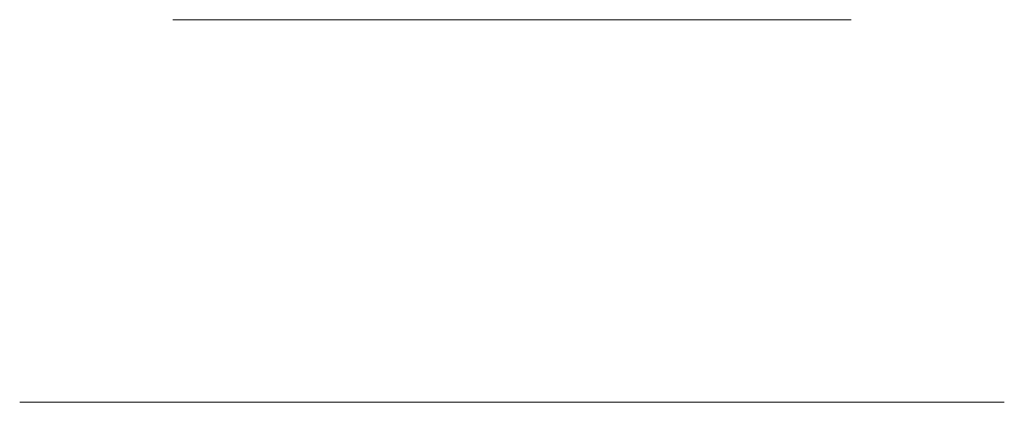
# Model space of a CAD drawing. Units: millimetres. Extents: x 481.8 to 571.8, y 0 to 35.
import ezdxf

# ---------------------------------------------------------------- set-up
doc = ezdxf.new("R2010")
doc.units = ezdxf.units.MM
doc.layers.add('M-CONS', color=8, linetype='Continuous', lineweight=18)

msp = doc.modelspace()

# ---------------------------------------------------------------- linework, layer by layer
at = {"layer": 'M-CONS', "extrusion": (0, -1, 0), "elevation": -35}
msp.add_lwpolyline([(557.838, 188.085), (557.838, 165.704, 0.399387), (495.838, 165.704), (495.838, 188.085), (526.838, 188.085)], format="xyb", close=True, dxfattribs=at)
at = {"layer": 'M-CONS', "extrusion": (0, -1, 0)}
msp.add_lwpolyline([(526.838, 156.416), (517.838, 156.416), (517.838, 149.277, 4.20673), (535.838, 149.277), (535.838, 156.416)], format="xyb", close=True, dxfattribs=at)
for centre, radius in [((526.838, 133.085), 45), ((526.838, 131.416), 35)]:
    msp.add_circle(centre, radius, dxfattribs=at)

doc.saveas('drawing.dxf')
